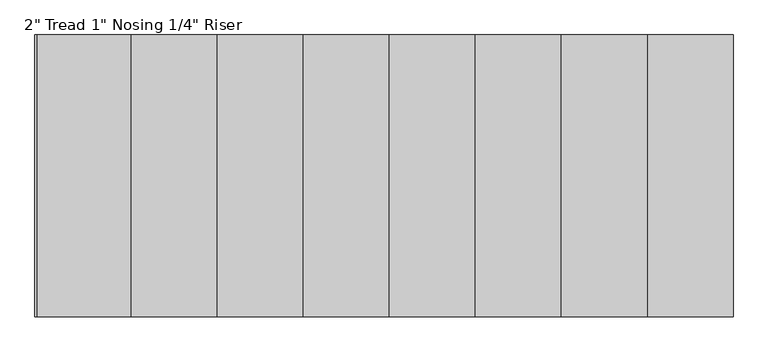
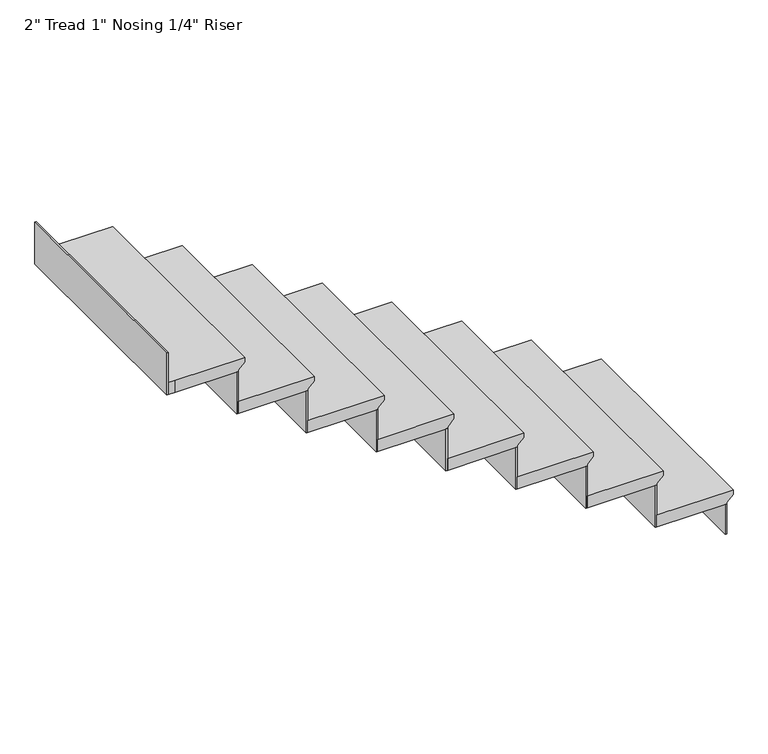
"""IFC4 building model written with IfcOpenShell, lengths in millimetres: stair flight geometry."""

from ifc_helpers import new_model, si_unit, origin, place, context, project, spatial, faceted_brep, source, transform, mapped, element, save


def stair_flight_ae0811cb(model_context):
    return source(origin(), model_context, "Body", "Brep", [
        faceted_brep([(-4313.7591614, 371.2049437, 3359.15), (-4313.7591614, 371.2049437, 3378.2), (-4313.7591614, -543.1950563, 3378.2), (-4313.7591614, -543.1950563, 3359.15), (-4339.1591614, 371.2049437, 3333.75), (-4339.1591614, -543.1950563, 3333.75), (-4618.5591614, 371.2049437, 3378.2), (-4618.5591614, -543.1950563, 3378.2), (-4339.1591614, -543.1950563, 3327.4), (-4618.5591614, -543.1950563, 3327.4), (-4618.5591614, 371.2049437, 3327.4), (-4339.1591614, 371.2049437, 3327.4)], [[[0, 1, 2, 3]], [[4, 0, 3, 5]], [[2, 1, 6, 7]], [[8, 9, 10, 11]], [[2, 7, 9, 8, 5, 3]], [[8, 11, 4, 5]], [[6, 1, 0, 4, 11, 10]], [[7, 6, 10, 9]]]),
        faceted_brep([(-4339.1591614, 371.2049437, 3327.4), (-4339.1591614, 371.2049437, 3200.4), (-4345.5091614, 371.2049437, 3200.4), (-4345.5091614, 371.2049437, 3327.4), (-4339.1591614, -543.1950563, 3327.4), (-4345.5091614, -543.1950563, 3327.4), (-4345.5091614, -543.1950563, 3200.4), (-4339.1591614, -543.1950563, 3200.4)], [[[0, 1, 2, 3]], [[4, 5, 6, 7]], [[1, 0, 4, 7]], [[2, 1, 7, 6]], [[3, 2, 6, 5]], [[0, 3, 5, 4]]]),
        faceted_brep([(-4618.5591614, 371.2049437, 3505.2), (-4618.5591614, 371.2049437, 3327.4), (-4624.9091614, 371.2049437, 3327.4), (-4624.9091614, 371.2049437, 3505.2), (-4618.5591614, -543.1950563, 3505.2), (-4624.9091614, -543.1950563, 3505.2), (-4624.9091614, -543.1950563, 3327.4), (-4618.5591614, -543.1950563, 3327.4)], [[[0, 1, 2, 3]], [[4, 5, 6, 7]], [[1, 0, 4, 7]], [[2, 1, 7, 6]], [[3, 2, 6, 5]], [[0, 3, 5, 4]]]),
        faceted_brep([(-4593.1591614, -543.1950563, 3556.0), (-4593.1591614, 371.2049437, 3556.0), (-4897.9591614, 371.2049437, 3556.0), (-4897.9591614, -543.1950563, 3556.0), (-4618.5591614, -543.1950563, 3505.2), (-4897.9591614, -543.1950563, 3505.2), (-4897.9591614, 371.2049437, 3505.2), (-4618.5591614, 371.2049437, 3505.2), (-4618.5591614, -543.1950563, 3511.55), (-4593.1591614, -543.1950563, 3536.95), (-4618.5591614, 371.2049437, 3511.55), (-4593.1591614, 371.2049437, 3536.95)], [[[0, 1, 2, 3]], [[4, 5, 6, 7]], [[0, 3, 5, 4, 8, 9]], [[4, 7, 10, 8]], [[2, 1, 11, 10, 7, 6]], [[3, 2, 6, 5]], [[11, 1, 0, 9]], [[10, 11, 9, 8]]]),
        faceted_brep([(-4897.9591614, 371.2049437, 3683.0), (-4897.9591614, 371.2049437, 3505.2), (-4904.3091614, 371.2049437, 3505.2), (-4904.3091614, 371.2049437, 3683.0), (-4897.9591614, -543.1950563, 3683.0), (-4904.3091614, -543.1950563, 3683.0), (-4904.3091614, -543.1950563, 3505.2), (-4897.9591614, -543.1950563, 3505.2)], [[[0, 1, 2, 3]], [[4, 5, 6, 7]], [[1, 0, 4, 7]], [[2, 1, 7, 6]], [[3, 2, 6, 5]], [[0, 3, 5, 4]]]),
        faceted_brep([(-4872.5591614, -543.1950563, 3733.8), (-4872.5591614, 371.2049437, 3733.8), (-5177.3591614, 371.2049437, 3733.8), (-5177.3591614, -543.1950563, 3733.8), (-4897.9591614, -543.1950563, 3683.0), (-5177.3591614, -543.1950563, 3683.0), (-5177.3591614, 371.2049437, 3683.0), (-4897.9591614, 371.2049437, 3683.0), (-4897.9591614, -543.1950563, 3689.35), (-4872.5591614, -543.1950563, 3714.75), (-4897.9591614, 371.2049437, 3689.35), (-4872.5591614, 371.2049437, 3714.75)], [[[0, 1, 2, 3]], [[4, 5, 6, 7]], [[0, 3, 5, 4, 8, 9]], [[4, 7, 10, 8]], [[2, 1, 11, 10, 7, 6]], [[3, 2, 6, 5]], [[11, 1, 0, 9]], [[10, 11, 9, 8]]]),
        faceted_brep([(-5177.3591614, 371.2049437, 3860.8), (-5177.3591614, 371.2049437, 3683.0), (-5183.7091614, 371.2049437, 3683.0), (-5183.7091614, 371.2049437, 3860.8), (-5177.3591614, -543.1950563, 3860.8), (-5183.7091614, -543.1950563, 3860.8), (-5183.7091614, -543.1950563, 3683.0), (-5177.3591614, -543.1950563, 3683.0)], [[[0, 1, 2, 3]], [[4, 5, 6, 7]], [[1, 0, 4, 7]], [[2, 1, 7, 6]], [[3, 2, 6, 5]], [[0, 3, 5, 4]]]),
        faceted_brep([(-5151.9591614, -543.1950563, 3911.6), (-5151.9591614, 371.2049437, 3911.6), (-5456.7591614, 371.2049437, 3911.6), (-5456.7591614, -543.1950563, 3911.6), (-5177.3591614, -543.1950563, 3860.8), (-5456.7591614, -543.1950563, 3860.8), (-5456.7591614, 371.2049437, 3860.8), (-5177.3591614, 371.2049437, 3860.8), (-5177.3591614, -543.1950563, 3867.15), (-5151.9591614, -543.1950563, 3892.55), (-5177.3591614, 371.2049437, 3867.15), (-5151.9591614, 371.2049437, 3892.55)], [[[0, 1, 2, 3]], [[4, 5, 6, 7]], [[0, 3, 5, 4, 8, 9]], [[4, 7, 10, 8]], [[2, 1, 11, 10, 7, 6]], [[3, 2, 6, 5]], [[11, 1, 0, 9]], [[10, 11, 9, 8]]]),
        faceted_brep([(-5456.7591614, 371.2049437, 4038.6), (-5456.7591614, 371.2049437, 3860.8), (-5463.1091614, 371.2049437, 3860.8), (-5463.1091614, 371.2049437, 4038.6), (-5456.7591614, -543.1950563, 4038.6), (-5463.1091614, -543.1950563, 4038.6), (-5463.1091614, -543.1950563, 3860.8), (-5456.7591614, -543.1950563, 3860.8)], [[[0, 1, 2, 3]], [[4, 5, 6, 7]], [[1, 0, 4, 7]], [[2, 1, 7, 6]], [[3, 2, 6, 5]], [[0, 3, 5, 4]]]),
        faceted_brep([(-5431.3591614, -543.1950563, 4089.4), (-5431.3591614, 371.2049437, 4089.4), (-5736.1591614, 371.2049437, 4089.4), (-5736.1591614, -543.1950563, 4089.4), (-5456.7591614, -543.1950563, 4038.6), (-5736.1591614, -543.1950563, 4038.6), (-5736.1591614, 371.2049437, 4038.6), (-5456.7591614, 371.2049437, 4038.6), (-5456.7591614, -543.1950563, 4044.95), (-5431.3591614, -543.1950563, 4070.35), (-5456.7591614, 371.2049437, 4044.95), (-5431.3591614, 371.2049437, 4070.35)], [[[0, 1, 2, 3]], [[4, 5, 6, 7]], [[0, 3, 5, 4, 8, 9]], [[4, 7, 10, 8]], [[2, 1, 11, 10, 7, 6]], [[3, 2, 6, 5]], [[11, 1, 0, 9]], [[10, 11, 9, 8]]]),
        faceted_brep([(-5736.1591614, 371.2049437, 4216.4), (-5736.1591614, 371.2049437, 4038.6), (-5742.5091614, 371.2049437, 4038.6), (-5742.5091614, 371.2049437, 4216.4), (-5736.1591614, -543.1950563, 4216.4), (-5742.5091614, -543.1950563, 4216.4), (-5742.5091614, -543.1950563, 4038.6), (-5736.1591614, -543.1950563, 4038.6)], [[[0, 1, 2, 3]], [[4, 5, 6, 7]], [[1, 0, 4, 7]], [[2, 1, 7, 6]], [[3, 2, 6, 5]], [[0, 3, 5, 4]]]),
        faceted_brep([(-5710.7591614, -543.1950563, 4267.2), (-5710.7591614, 371.2049437, 4267.2), (-6015.5591614, 371.2049437, 4267.2), (-6015.5591614, -543.1950563, 4267.2), (-5736.1591614, -543.1950563, 4216.4), (-6015.5591614, -543.1950563, 4216.4), (-6015.5591614, 371.2049437, 4216.4), (-5736.1591614, 371.2049437, 4216.4), (-5736.1591614, -543.1950563, 4222.75), (-5710.7591614, -543.1950563, 4248.15), (-5736.1591614, 371.2049437, 4222.75), (-5710.7591614, 371.2049437, 4248.15)], [[[0, 1, 2, 3]], [[4, 5, 6, 7]], [[0, 3, 5, 4, 8, 9]], [[4, 7, 10, 8]], [[2, 1, 11, 10, 7, 6]], [[3, 2, 6, 5]], [[11, 1, 0, 9]], [[10, 11, 9, 8]]]),
        faceted_brep([(-6015.5591614, 371.2049437, 4394.2), (-6015.5591614, 371.2049437, 4216.4), (-6021.9091614, 371.2049437, 4216.4), (-6021.9091614, 371.2049437, 4394.2), (-6015.5591614, -543.1950563, 4394.2), (-6021.9091614, -543.1950563, 4394.2), (-6021.9091614, -543.1950563, 4216.4), (-6015.5591614, -543.1950563, 4216.4)], [[[0, 1, 2, 3]], [[4, 5, 6, 7]], [[1, 0, 4, 7]], [[2, 1, 7, 6]], [[3, 2, 6, 5]], [[0, 3, 5, 4]]]),
        faceted_brep([(-5990.1591614, -543.1950563, 4445.0), (-5990.1591614, 371.2049437, 4445.0), (-6294.9591614, 371.2049437, 4445.0), (-6294.9591614, -543.1950563, 4445.0), (-6015.5591614, -543.1950563, 4394.2), (-6294.9591614, -543.1950563, 4394.2), (-6294.9591614, 371.2049437, 4394.2), (-6015.5591614, 371.2049437, 4394.2), (-6015.5591614, -543.1950563, 4400.55), (-5990.1591614, -543.1950563, 4425.95), (-6015.5591614, 371.2049437, 4400.55), (-5990.1591614, 371.2049437, 4425.95)], [[[0, 1, 2, 3]], [[4, 5, 6, 7]], [[0, 3, 5, 4, 8, 9]], [[4, 7, 10, 8]], [[2, 1, 11, 10, 7, 6]], [[3, 2, 6, 5]], [[11, 1, 0, 9]], [[10, 11, 9, 8]]]),
        faceted_brep([(-6574.3591614, 371.2049437, 4749.8), (-6574.3591614, 371.2049437, 4572.0), (-6580.7091614, 371.2049437, 4572.0), (-6580.7091614, 371.2049437, 4749.8), (-6574.3591614, -543.1950563, 4749.8), (-6580.7091614, -543.1950563, 4749.8), (-6580.7091614, -543.1950563, 4572.0), (-6574.3591614, -543.1950563, 4572.0)], [[[0, 1, 2, 3]], [[4, 5, 6, 7]], [[1, 0, 4, 7]], [[2, 1, 7, 6]], [[3, 2, 6, 5]], [[0, 3, 5, 4]]]),
        faceted_brep([(-6294.9591614, 371.2049437, 4572.0), (-6294.9591614, 371.2049437, 4394.2), (-6301.3091614, 371.2049437, 4394.2), (-6301.3091614, 371.2049437, 4572.0), (-6294.9591614, -543.1950563, 4572.0), (-6301.3091614, -543.1950563, 4572.0), (-6301.3091614, -543.1950563, 4394.2), (-6294.9591614, -543.1950563, 4394.2)], [[[0, 1, 2, 3]], [[4, 5, 6, 7]], [[1, 0, 4, 7]], [[2, 1, 7, 6]], [[3, 2, 6, 5]], [[0, 3, 5, 4]]]),
        faceted_brep([(-6574.3591614, -543.1950563, 4622.8), (-6548.9591614, -543.1950563, 4622.8), (-6269.5591614, -543.1950563, 4622.8), (-6269.5591614, 371.2049437, 4622.8), (-6574.3591614, 371.2049437, 4622.8), (-6548.9591614, -543.1950563, 4572.0), (-6574.3591614, -543.1950563, 4572.0), (-6574.3591614, 371.2049437, 4572.0), (-6294.9591614, 371.2049437, 4572.0), (-6294.9591614, -543.1950563, 4572.0), (-6294.9591614, -543.1950563, 4578.35), (-6269.5591614, -543.1950563, 4603.75), (-6294.9591614, 371.2049437, 4578.35), (-6269.5591614, 371.2049437, 4603.75)], [[[0, 1, 2, 3, 4]], [[5, 6, 7, 8, 9]], [[1, 0, 6, 5]], [[2, 1, 5, 9, 10, 11]], [[9, 8, 12, 10]], [[4, 3, 13, 12, 8, 7]], [[0, 4, 7, 6]], [[13, 3, 2, 11]], [[12, 13, 11, 10]]]),
    ])


if __name__ == "__main__":
    model = new_model("IFC4")
    model_context = context("Model", 3, world=origin())
    ifc_project = project(units=[si_unit("LENGTHUNIT", "METRE", prefix="MILLI")], contexts=[model_context])
    site = spatial("IfcSite", under=ifc_project)
    building = spatial("IfcBuilding", under=site)
    placement = place(None, origin())
    stair_flight_shape = stair_flight_ae0811cb(model_context)
    element("IfcStairFlight", 1, ObjectType="2\" Tread 1\" Nosing 1/4\" Riser", at=placement, inside=building, context=model_context, shape_type="MappedRepresentation", body=[
        mapped(stair_flight_shape, transform((0.0, 0.0, 0.0), x_axis=(1.0, 0.0, 0.0), y_axis=(0.0, 1.0, 0.0), z_axis=(0.0, 0.0, 1.0))),
    ])
    save(model, "model.ifc")
